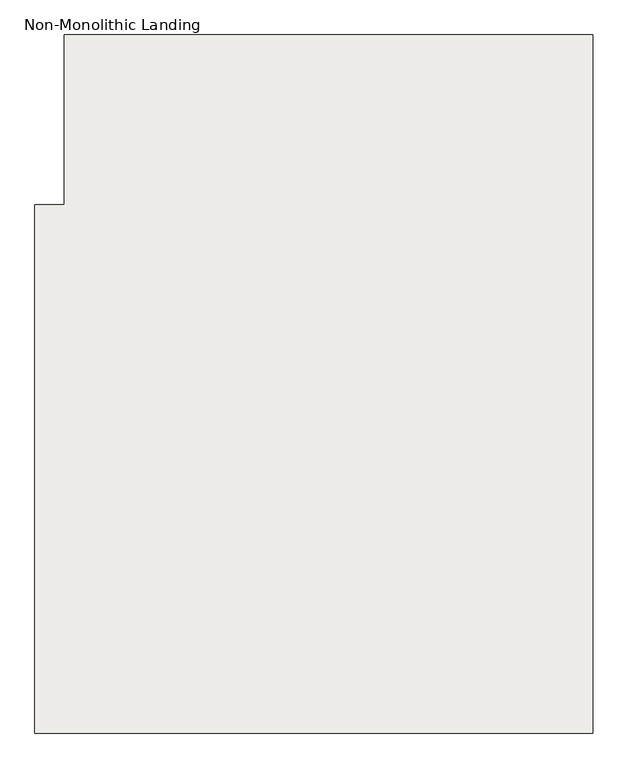
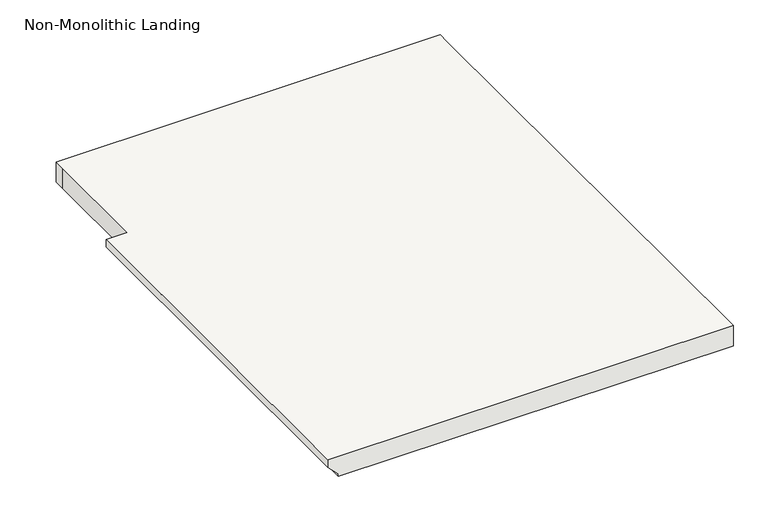
"""IFC4 building model written with IfcOpenShell, lengths in millimetres: slab geometry, Non-Monolithic Landing."""

from ifc_helpers import new_model, si_unit, origin, place, context, project, spatial, faceted_brep, source, transform, mapped, element, save


def non_monolithic_landing_589093d1(model_context):
    return source(origin(), model_context, "Body", "Brep", [
        faceted_brep([(8906.0423568, -10720.6073314, 1039.7289474), (8906.0423568, -10720.6073314, 1058.7789474), (8906.0423568, -9806.2073314, 1058.7789474), (8906.0423568, -9806.2073314, 1039.7289474), (8931.4423568, -10720.6073314, 1014.3289474), (8931.4423568, -9806.2073314, 1014.3289474), (9871.2423568, -10720.6073314, 1058.7789474), (9871.2423568, -9537.7746824, 1058.7789474), (9871.2423568, -9512.3746824, 1058.7789474), (8956.8423568, -9512.3746824, 1058.7789474), (8956.8423568, -9537.7746824, 1058.7789474), (8956.8423568, -9806.2073314, 1058.7789474), (8931.4423568, -10720.6073314, 1007.9789474), (8931.4423568, -9806.2073314, 1007.9789474), (8956.8423568, -9806.2073314, 1007.9789474), (8956.8423568, -9537.7746824, 1007.9789474), (8956.8423568, -9512.3746824, 1007.9789474), (9871.2423568, -9512.3746824, 1007.9789474), (9871.2423568, -9537.7746824, 1007.9789474), (9871.2423568, -10720.6073314, 1007.9789474)], [[[0, 1, 2, 3]], [[4, 0, 3, 5]], [[6, 7, 8, 9, 10, 11, 2, 1]], [[12, 13, 14, 15, 16, 17, 18, 19]], [[13, 12, 4, 5]], [[6, 1, 0, 4, 12, 19]], [[7, 6, 19, 18]], [[8, 7, 18, 17]], [[9, 8, 17, 16]], [[10, 9, 16, 15]], [[11, 10, 15, 14]], [[2, 11, 14, 13, 5, 3]]]),
    ])


if __name__ == "__main__":
    model = new_model("IFC4")
    model_context = context("Model", 3, world=origin())
    ifc_project = project(units=[si_unit("LENGTHUNIT", "METRE", prefix="MILLI")], contexts=[model_context])
    site = spatial("IfcSite", under=ifc_project)
    building = spatial("IfcBuilding", under=site)
    placement = place(None, origin())
    non_monolithic_landing_shape = non_monolithic_landing_589093d1(model_context)
    element("IfcSlab", 1, ObjectType="Non-Monolithic Landing", at=placement, inside=building, context=model_context, shape_type="MappedRepresentation", body=[
        mapped(non_monolithic_landing_shape, transform((0.0, 0.0, 0.0), x_axis=(1.0, 0.0, 0.0), y_axis=(0.0, 1.0, 0.0), z_axis=(0.0, 0.0, 1.0))),
    ])
    save(model, "model.ifc")

# Revit data of these elements
# Element 1 (IfcSlab, "Non-Monolithic Landing")
#   Materials on its faces: "MARBLE STAIRS 6\""
# Materials
#   "MARBLE STAIRS 6\"": class "Generic", colour RGB 120 120 120, transparency 0, Cost = 0
